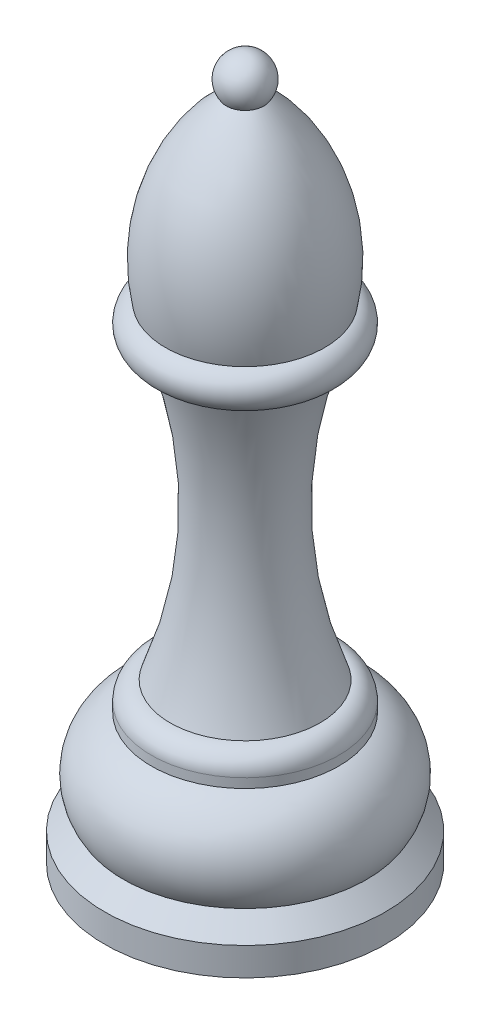
ISO-10303-21;
HEADER;
FILE_DESCRIPTION(('STEP AP214'),'2;1');
FILE_NAME('part.step','',(''),(''),'','','');
FILE_SCHEMA(('AUTOMOTIVE_DESIGN { 1 0 10303 214 1 1 1 1 }'));
ENDSEC;
DATA;
#1=APPLICATION_CONTEXT('core data for automotive mechanical design processes');
#2=APPLICATION_PROTOCOL_DEFINITION('international standard','automotive_design',2000,#1);
#3=PRODUCT_CONTEXT('',#1,'mechanical');
#4=PRODUCT('Part','Part','',(#3));
#5=PRODUCT_RELATED_PRODUCT_CATEGORY('part','',(#4));
#6=PRODUCT_DEFINITION_FORMATION('','',#4);
#7=PRODUCT_DEFINITION_CONTEXT('part definition',#1,'design');
#8=PRODUCT_DEFINITION('design','',#6,#7);
#9=PRODUCT_DEFINITION_SHAPE('','',#8);
#10=(LENGTH_UNIT() NAMED_UNIT(*) SI_UNIT(.MILLI.,.METRE.));
#11=(NAMED_UNIT(*) PLANE_ANGLE_UNIT() SI_UNIT($,.RADIAN.));
#12=(NAMED_UNIT(*) SI_UNIT($,.STERADIAN.) SOLID_ANGLE_UNIT());
#13=UNCERTAINTY_MEASURE_WITH_UNIT(LENGTH_MEASURE(1.E-05),#10,'distance_accuracy_value','');
#14=(GEOMETRIC_REPRESENTATION_CONTEXT(3) GLOBAL_UNCERTAINTY_ASSIGNED_CONTEXT((#13)) GLOBAL_UNIT_ASSIGNED_CONTEXT((#10,
#11,#12)) REPRESENTATION_CONTEXT('',''));
#15=CARTESIAN_POINT('',(0.,0.,0.));
#16=DIRECTION('',(0.,0.,1.));
#17=DIRECTION('',(1.,0.,0.));
#18=AXIS2_PLACEMENT_3D('',#15,#16,#17);
#19=CARTESIAN_POINT('',(0.,0.,0.));
#20=DIRECTION('',(0.,-1.,0.));
#21=DIRECTION('',(0.,0.,-1.));
#22=AXIS2_PLACEMENT_3D('',#19,#20,#21);
#23=PLANE('',#22);
#24=CARTESIAN_POINT('',(0.,0.,0.));
#25=DIRECTION('',(0.,-1.,0.));
#26=DIRECTION('',(0.,0.,-1.));
#27=AXIS2_PLACEMENT_3D('',#24,#25,#26);
#28=CIRCLE('',#27,15.);
#29=CARTESIAN_POINT('',(0.,0.,-15.));
#30=VERTEX_POINT('',#29);
#31=EDGE_CURVE('E66',#30,#30,#28,.T.);
#32=ORIENTED_EDGE('',*,*,#31,.T.);
#33=EDGE_LOOP('',(#32));
#34=FACE_BOUND('',#33,.T.);
#35=ADVANCED_FACE('F40',(#34),#23,.T.);
#36=CARTESIAN_POINT('',(0.,72.5,0.));
#37=DIRECTION('',(0.,-1.,0.));
#38=DIRECTION('',(1.,0.,0.));
#39=AXIS2_PLACEMENT_3D('',#36,#37,#38);
#40=SPHERICAL_SURFACE('',#39,2.5);
#41=CARTESIAN_POINT('',(0.,71.,0.));
#42=DIRECTION('',(0.,-1.,0.));
#43=DIRECTION('',(0.,0.,-1.));
#44=AXIS2_PLACEMENT_3D('',#41,#42,#43);
#45=CIRCLE('',#44,2.);
#46=CARTESIAN_POINT('',(0.,71.,-2.));
#47=VERTEX_POINT('',#46);
#48=EDGE_CURVE('E10',#47,#47,#45,.T.);
#49=ORIENTED_EDGE('',*,*,#48,.F.);
#50=EDGE_LOOP('',(#49));
#51=FACE_BOUND('',#50,.T.);
#52=ADVANCED_FACE('F82',(#51),#40,.T.);
#53=CARTESIAN_POINT('',(0.,55.8883209789195,0.));
#54=DIRECTION('',(0.,-1.,0.));
#55=DIRECTION('',(0.,0.,-1.));
#56=AXIS2_PLACEMENT_3D('',#53,#54,#55);
#57=DEGENERATE_TOROIDAL_SURFACE('',#56,11.1010364919664,20.,.F.);
#58=ORIENTED_EDGE('',*,*,#48,.T.);
#59=EDGE_LOOP('',(#58));
#60=FACE_BOUND('',#59,.T.);
#61=CARTESIAN_POINT('',(0.,51.9134790398478,0.));
#62=DIRECTION('',(0.,-1.,0.));
#63=DIRECTION('',(0.,0.,-1.));
#64=AXIS2_PLACEMENT_3D('',#61,#62,#63);
#65=CIRCLE('',#64,8.5);
#66=CARTESIAN_POINT('',(0.,51.9134790398478,-8.5));
#67=VERTEX_POINT('',#66);
#68=EDGE_CURVE('E43',#67,#67,#65,.T.);
#69=ORIENTED_EDGE('',*,*,#68,.F.);
#70=EDGE_LOOP('',(#69));
#71=FACE_BOUND('',#70,.T.);
#72=ADVANCED_FACE('F87',(#60,#71),#57,.F.);
#73=CARTESIAN_POINT('',(0.,49.951789259375,0.));
#74=DIRECTION('',(0.,-1.,0.));
#75=DIRECTION('',(0.,0.,-1.));
#76=AXIS2_PLACEMENT_3D('',#73,#74,#75);
#77=TOROIDAL_SURFACE('',#76,7.96725773506285,2.03274226493715);
#78=ORIENTED_EDGE('',*,*,#68,.T.);
#79=EDGE_LOOP('',(#78));
#80=FACE_BOUND('',#79,.T.);
#81=CARTESIAN_POINT('',(0.,47.9734790398478,0.));
#82=DIRECTION('',(0.,-1.,0.));
#83=DIRECTION('',(0.,0.,-1.));
#84=AXIS2_PLACEMENT_3D('',#81,#82,#83);
#85=CIRCLE('',#84,7.5);
#86=CARTESIAN_POINT('',(0.,47.9734790398478,-7.5));
#87=VERTEX_POINT('',#86);
#88=EDGE_CURVE('E50',#87,#87,#85,.T.);
#89=ORIENTED_EDGE('',*,*,#88,.F.);
#90=EDGE_LOOP('',(#89));
#91=FACE_BOUND('',#90,.T.);
#92=ADVANCED_FACE('F92',(#80,#91),#77,.T.);
#93=CARTESIAN_POINT('',(0.,33.1547704586982,0.));
#94=DIRECTION('',(0.,-1.,0.));
#95=DIRECTION('',(0.,0.,-1.));
#96=AXIS2_PLACEMENT_3D('',#93,#94,#95);
#97=TOROIDAL_SURFACE('',#96,49.9900679687261,45.);
#98=ORIENTED_EDGE('',*,*,#88,.T.);
#99=EDGE_LOOP('',(#98));
#100=FACE_BOUND('',#99,.T.);
#101=CARTESIAN_POINT('',(0.,16.9734790398478,0.));
#102=DIRECTION('',(0.,-1.,0.));
#103=DIRECTION('',(0.,0.,-1.));
#104=AXIS2_PLACEMENT_3D('',#101,#102,#103);
#105=CIRCLE('',#104,8.);
#106=CARTESIAN_POINT('',(0.,16.9734790398478,-8.));
#107=VERTEX_POINT('',#106);
#108=EDGE_CURVE('E51',#107,#107,#105,.T.);
#109=ORIENTED_EDGE('',*,*,#108,.F.);
#110=EDGE_LOOP('',(#109));
#111=FACE_BOUND('',#110,.T.);
#112=ADVANCED_FACE('F98',(#100,#111),#97,.F.);
#113=CARTESIAN_POINT('',(0.,14.9734790398478,0.));
#114=DIRECTION('',(0.,-1.,0.));
#115=DIRECTION('',(0.,0.,-1.));
#116=AXIS2_PLACEMENT_3D('',#113,#114,#115);
#117=TOROIDAL_SURFACE('',#116,8.,2.);
#118=ORIENTED_EDGE('',*,*,#108,.T.);
#119=EDGE_LOOP('',(#118));
#120=FACE_BOUND('',#119,.T.);
#121=CARTESIAN_POINT('',(0.,14.9734790398478,0.));
#122=DIRECTION('',(0.,-1.,0.));
#123=DIRECTION('',(0.,0.,-1.));
#124=AXIS2_PLACEMENT_3D('',#121,#122,#123);
#125=CIRCLE('',#124,10.);
#126=CARTESIAN_POINT('',(0.,14.9734790398478,-10.));
#127=VERTEX_POINT('',#126);
#128=EDGE_CURVE('E57',#127,#127,#125,.T.);
#129=ORIENTED_EDGE('',*,*,#128,.F.);
#130=EDGE_LOOP('',(#129));
#131=FACE_BOUND('',#130,.T.);
#132=ADVANCED_FACE('F105',(#120,#131),#117,.T.);
#133=CARTESIAN_POINT('',(0.,0.,0.));
#134=DIRECTION('',(0.,-1.,0.));
#135=DIRECTION('',(0.,0.,-1.));
#136=AXIS2_PLACEMENT_3D('',#133,#134,#135);
#137=CYLINDRICAL_SURFACE('',#136,10.);
#138=ORIENTED_EDGE('',*,*,#128,.T.);
#139=EDGE_LOOP('',(#138));
#140=FACE_BOUND('',#139,.T.);
#141=CARTESIAN_POINT('',(0.,13.9734790398478,0.));
#142=DIRECTION('',(0.,-1.,0.));
#143=DIRECTION('',(0.,0.,-1.));
#144=AXIS2_PLACEMENT_3D('',#141,#142,#143);
#145=CIRCLE('',#144,10.);
#146=CARTESIAN_POINT('',(0.,13.9734790398478,-10.));
#147=VERTEX_POINT('',#146);
#148=EDGE_CURVE('E56',#147,#147,#145,.T.);
#149=ORIENTED_EDGE('',*,*,#148,.F.);
#150=EDGE_LOOP('',(#149));
#151=FACE_BOUND('',#150,.T.);
#152=ADVANCED_FACE('F108',(#140,#151),#137,.T.);
#153=CARTESIAN_POINT('',(0.,8.3166247903554,0.));
#154=DIRECTION('',(0.,-1.,0.));
#155=DIRECTION('',(0.,0.,-1.));
#156=AXIS2_PLACEMENT_3D('',#153,#154,#155);
#157=TOROIDAL_SURFACE('',#156,8.,6.);
#158=ORIENTED_EDGE('',*,*,#148,.T.);
#159=EDGE_LOOP('',(#158));
#160=FACE_BOUND('',#159,.T.);
#161=CARTESIAN_POINT('',(0.,5.,0.));
#162=DIRECTION('',(0.,-1.,0.));
#163=DIRECTION('',(0.,0.,-1.));
#164=AXIS2_PLACEMENT_3D('',#161,#162,#163);
#165=CIRCLE('',#164,13.);
#166=CARTESIAN_POINT('',(0.,5.,-13.));
#167=VERTEX_POINT('',#166);
#168=EDGE_CURVE('E65',#167,#167,#165,.T.);
#169=ORIENTED_EDGE('',*,*,#168,.F.);
#170=EDGE_LOOP('',(#169));
#171=FACE_BOUND('',#170,.T.);
#172=ADVANCED_FACE('F83',(#160,#171),#157,.T.);
#173=CARTESIAN_POINT('',(0.,3.,0.));
#174=DIRECTION('',(0.,-1.,0.));
#175=DIRECTION('',(0.,0.,-1.));
#176=AXIS2_PLACEMENT_3D('',#173,#174,#175);
#177=CONICAL_SURFACE('',#176,15.,0.785398163397449);
#178=ORIENTED_EDGE('',*,*,#168,.T.);
#179=EDGE_LOOP('',(#178));
#180=FACE_BOUND('',#179,.T.);
#181=CARTESIAN_POINT('',(0.,3.,0.));
#182=DIRECTION('',(0.,-1.,0.));
#183=DIRECTION('',(0.,0.,-1.));
#184=AXIS2_PLACEMENT_3D('',#181,#182,#183);
#185=CIRCLE('',#184,15.);
#186=CARTESIAN_POINT('',(0.,3.,-15.));
#187=VERTEX_POINT('',#186);
#188=EDGE_CURVE('E64',#187,#187,#185,.T.);
#189=ORIENTED_EDGE('',*,*,#188,.F.);
#190=EDGE_LOOP('',(#189));
#191=FACE_BOUND('',#190,.T.);
#192=ADVANCED_FACE('F74',(#180,#191),#177,.T.);
#193=CARTESIAN_POINT('',(0.,0.,0.));
#194=DIRECTION('',(0.,-1.,0.));
#195=DIRECTION('',(0.,0.,-1.));
#196=AXIS2_PLACEMENT_3D('',#193,#194,#195);
#197=CYLINDRICAL_SURFACE('',#196,15.);
#198=ORIENTED_EDGE('',*,*,#188,.T.);
#199=EDGE_LOOP('',(#198));
#200=FACE_BOUND('',#199,.T.);
#201=ORIENTED_EDGE('',*,*,#31,.F.);
#202=EDGE_LOOP('',(#201));
#203=FACE_BOUND('',#202,.T.);
#204=ADVANCED_FACE('F71',(#200,#203),#197,.T.);
#205=CLOSED_SHELL('',(#35,#52,#72,#92,#112,#132,#152,#172,#192,#204));
#206=MANIFOLD_SOLID_BREP('B2',#205);
#207=ADVANCED_BREP_SHAPE_REPRESENTATION('',(#18,#206),#14);
#208=SHAPE_DEFINITION_REPRESENTATION(#9,#207);
ENDSEC;
END-ISO-10303-21;
